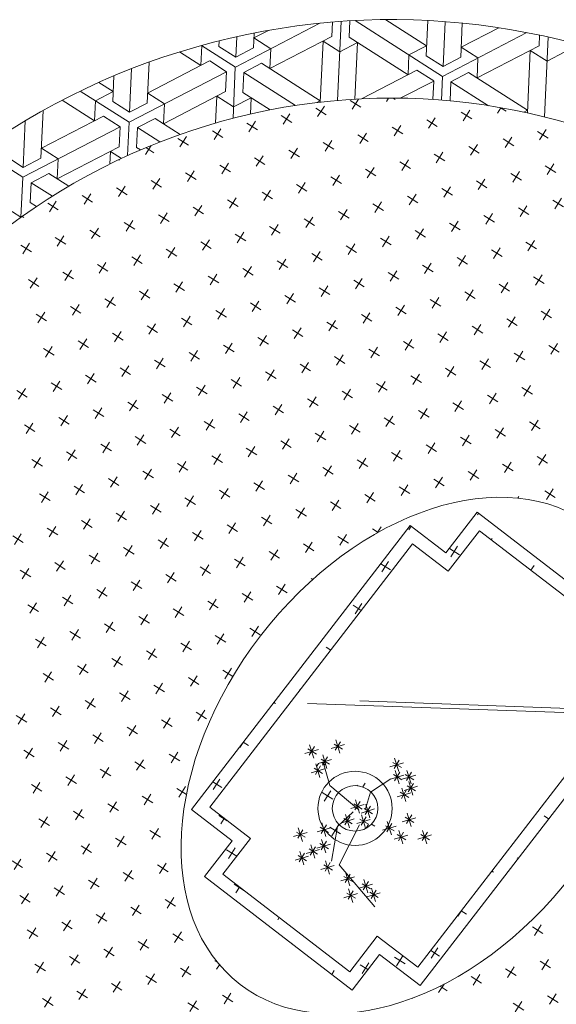
# Model space of a CAD drawing. Units: inches. Extents: x -4843 to -3402, y -164 to 3629.
# Tile 12 of 22: x -4506 to -4487, y 864 to 900. Entities that reach past the tile are written whole.
import ezdxf

# ---------------------------------------------------------------- set-up
doc = ezdxf.new("R2010")
doc.units = ezdxf.units.IN
doc.layers.add('furniture', color=6, linetype='Continuous', lineweight=18)

# ---------------------------------------------------------------- blocks, each defined once
blk = doc.blocks.new('A$C30AE1D3B')
for p, q in [((1385.7, 1569.4, -685.7), (1368.4, 1561.4, -685.7)), ((1381.1, 1556.7, -685.7), (1373, 1574, -685.7)), ((1436.3, 1551, -685.7), (1419.1, 1542.9, -685.7)), ((1431.7, 1538.3, -685.7), (1423.7, 1555.6, -685.7)), ((1362.7, 1506.1, -685.7), (1354.6, 1523.4, -685.7)), ((1367.3, 1518.8, -685.7), (1350, 1510.7, -685.7)), ((1413.3, 1487.7, -685.7), (1405.2, 1504.9, -685.7)), ((1417.9, 1500.3, -685.7), (1400.6, 1492.3, -685.7)), ((1468.5, 1481.9, -685.7), (1451.3, 1473.9, -685.7)), ((1463.9, 1469.3, -685.7), (1455.9, 1486.5, -685.7)), ((1348.8, 1468.1, -685.7), (1331.6, 1460.1, -685.7)), ((1344.2, 1455.5, -685.7), (1336.2, 1472.7, -685.7)), ((1519.2, 1463.5, -685.7), (1505.1, 1456.9, -685.7)), ((1512, 1456.3, -685.7), (1506.5, 1468.1, -685.7)), ((1557.3, 1449.2, -685.7), (1557.1, 1449.7, -685.7)), ((1013.2, 1248.8, -685.7), (1537, 1439.4, -685.7)), ((1537, 1439.4, -685.7), (1563.8, 1365.8, -685.7)), ((1494.9, 1402.8, -685.7), (1488.1, 1417.5, -685.7)), ((1038.9, 1236.8, -685.7), (1525.1, 1413.8, -685.7)), ((1500.7, 1412.9, -685.7), (1483.5, 1404.8, -685.7)), ((1525.1, 1413.8, -685.7), (1551.9, 1340.2, -685.7)), ((1423, 1376.7, -685.7), (1419, 1385.3, -685.7)), ((1551.4, 1394.4, -685.7), (1534.9, 1386.8, -685.7)), ((1546.8, 1381.8, -685.7), (1538.7, 1399, -685.7)), ((1563.8, 1365.8, -685.7), (1628.5, 1389.4, -685.7)), ((1628.5, 1389.4, -685.7), (1725.8, 1122.2, -685.7)), ((1431.7, 1380.6, -685.7), (1423.4, 1376.8, -685.7)), ((1602, 1376, -685.7), (1584.7, 1367.9, -685.7)), ((1597.4, 1363.3, -685.7), (1591.5, 1375.9, -685.7)), ((1307.4, 1354.2, -685.7), (1306.7, 1355.6, -685.7)), ((1551.9, 1340.2, -685.7), (1616.6, 1363.7, -685.7)), ((1616.6, 1363.7, -685.7), (1700.1, 1134.1, -685.7)), ((1351.1, 1350.5, -685.7), (1349.9, 1353.1, -685.7)), ((1641.9, 1352.6, -685.7), (1635.4, 1349.5, -685.7)), ((1238.3, 1322, -685.7), (1234.8, 1329.4, -685.7)), ((1525.7, 1294.5, -685.7), (1520, 1273.8, -685.7)), ((1542.7, 1217.2, -685.7), (1530.9, 1300.7, -685.7)), ((1804.5, 1302.3, -685.7), (1787.3, 1294.2, -685.7)), ((1799.9, 1289.6, -685.7), (1791.9, 1306.9, -685.7)), ((1533.2, 1281.3, -685.7), (1512.5, 1287.1, -685.7)), ((1529.1, 1286.7, -685.7), (1515.5, 1280.1, -685.7)), ((1525.6, 1277.8, -685.7), (1518.9, 1291.5, -685.7)), ((1668.1, 1280.7, -685.7), (1667.6, 1280.5, -685.7)), ((1855.2, 1283.9, -685.7), (1837.9, 1275.8, -685.7)), ((1850.5, 1271.2, -685.7), (1842.5, 1288.5, -685.7)), ((1536.2, 1263.8, -685.7), (1515.5, 1269.5, -685.7)), ((1532.1, 1269.2, -685.7), (1518.5, 1262.5, -685.7)), ((1528.6, 1260.3, -685.7), (1521.9, 1274, -685.7)), ((1528.7, 1277, -685.7), (1523, 1256.3, -685.7)), ((1563.4, 1263.5, -685.7), (1542.7, 1269.2, -685.7)), ((1559.3, 1268.9, -685.7), (1545.7, 1262.3, -685.7)), ((1555.8, 1260, -685.7), (1549.1, 1273.7, -685.7)), ((1555.9, 1276.7, -685.7), (1550.2, 1256, -685.7)), ((1419.9, 1248.5, -685.7), (1399.2, 1254.3, -685.7)), ((1415.8, 1254, -685.7), (1402.1, 1247.3, -685.7)), ((1412.3, 1245.1, -685.7), (1405.6, 1258.7, -685.7)), ((1412.4, 1261.8, -685.7), (1406.7, 1241.1, -685.7)), ((1545.9, 1236.1, -685.7), (1539.2, 1249.8, -685.7)), ((1546, 1252.8, -685.7), (1540.3, 1232.1, -685.7)), ((1786.1, 1251.6, -685.7), (1778.7, 1248.2, -685.7)), ((1381.8, 1022.6, -685.7), (1059.1, 1244.3, -685.7)), ((1450.6, 1229.2, -685.7), (1429.9, 1235, -685.7)), ((1446.5, 1234.7, -685.7), (1432.9, 1228, -685.7)), ((1443, 1225.7, -685.7), (1436.3, 1239.4, -685.7)), ((1443.1, 1242.4, -685.7), (1437.4, 1221.7, -685.7)), ((1553.5, 1239.5, -685.7), (1532.8, 1245.3, -685.7)), ((1549.4, 1245, -685.7), (1535.8, 1238.3, -685.7)), ((1666.4, 1237.9, -685.7), (1663, 1236.3, -685.7)), ((1781.5, 1239, -685.7), (1779.2, 1243.9, -685.7)), ((1832.1, 1220.6, -685.7), (1824.1, 1237.8, -685.7)), ((1425.9, 1213.4, -685.7), (1405.2, 1219.2, -685.7)), ((1421.8, 1218.9, -685.7), (1408.1, 1212.2, -685.7)), ((1418.3, 1210, -685.7), (1411.6, 1223.6, -685.7)), ((1418.4, 1226.7, -685.7), (1412.7, 1206, -685.7)), ((1450.8, 1221.5, -685.7), (1445, 1200.8, -685.7)), ((1562.5, 1221.5, -685.7), (1556.7, 1200.8, -685.7)), ((1836.7, 1233.2, -685.7), (1819.5, 1225.2, -685.7)), ((1882.7, 1202.1, -685.7), (1874.7, 1219.4, -685.7)), ((1451, 983.2, -685.7), (1128.3, 1204.9, -685.7)), ((1458.2, 1208.3, -685.7), (1437.5, 1214, -685.7)), ((1454.2, 1213.7, -685.7), (1440.5, 1207, -685.7)), ((1450.6, 1204.8, -685.7), (1444, 1218.5, -685.7)), ((1483.6, 1182.4, -685.7), (1542.7, 1217.2, -685.7)), ((1513.3, 1166.6, -685.7), (1549.3, 1206.3, -685.7)), ((1570, 1208.3, -685.7), (1549.3, 1214, -685.7)), ((1565.9, 1213.7, -685.7), (1552.2, 1207, -685.7)), ((1562.4, 1204.8, -685.7), (1555.7, 1218.5, -685.7)), ((1887.4, 1214.8, -685.7), (1870.1, 1206.7, -685.7)), ((1404.6, 1190.3, -685.7), (1398.8, 1169.6, -685.7)), ((1467.5, 1191.1, -685.7), (1465, 1196.5, -685.7)), ((1477.6, 1191.9, -685.7), (1471.6, 1189.1, -685.7)), ((1478.4, 1175.1, -685.7), (1471.7, 1188.8, -685.7)), ((1478.5, 1191.8, -685.7), (1472.8, 1171.1, -685.7)), ((1550, 1190.7, -685.7), (1544.3, 1170, -685.7)), ((1568.4, 1188.9, -685.7), (1562.7, 1168.2, -685.7)), ((1938, 1196.4, -685.7), (1920.7, 1188.3, -685.7)), ((1933.4, 1183.7, -685.7), (1925.3, 1201, -685.7)), ((1397.8, 1174.4, -685.7), (1377.1, 1180.2, -685.7)), ((1393.7, 1179.8, -685.7), (1380, 1173.2, -685.7)), ((1390.2, 1170.9, -685.7), (1383.5, 1184.6, -685.7)), ((1390.3, 1187.6, -685.7), (1384.6, 1166.9, -685.7)), ((1412, 1177.1, -685.7), (1391.3, 1182.8, -685.7)), ((1408, 1182.5, -685.7), (1394.3, 1175.8, -685.7)), ((1404.4, 1173.6, -685.7), (1397.8, 1187.3, -685.7)), ((1471.9, 1168.3, -685.7), (1451.2, 1174.1, -685.7)), ((1467.8, 1173.8, -685.7), (1454.2, 1167.1, -685.7)), ((1464.3, 1164.9, -685.7), (1457.6, 1178.6, -685.7)), ((1464.4, 1181.6, -685.7), (1458.7, 1160.9, -685.7)), ((1486, 1178.5, -685.7), (1465.3, 1184.3, -685.7)), ((1481.9, 1184, -685.7), (1468.2, 1177.3, -685.7)), ((1498.6, 1161.3, -685.7), (1492, 1174.9, -685.7)), ((1498.8, 1178, -685.7), (1493, 1157.3, -685.7)), ((1523.7, 1160.8, -685.7), (1515.6, 1178.1, -685.7)), ((1557.5, 1177.5, -685.7), (1536.8, 1183.2, -685.7)), ((1553.4, 1182.9, -685.7), (1539.7, 1176.2, -685.7)), ((1549.9, 1174, -685.7), (1543.2, 1187.7, -685.7)), ((1575.9, 1175.7, -685.7), (1555.2, 1181.5, -685.7)), ((1571.8, 1181.1, -685.7), (1558.2, 1174.5, -685.7)), ((1568.3, 1172.2, -685.7), (1561.6, 1185.9, -685.7)), ((1595.5, 1175.2, -685.7), (1574.8, 1181, -685.7)), ((1591.5, 1180.7, -685.7), (1577.8, 1174, -685.7)), ((1587.9, 1171.8, -685.7), (1581.3, 1185.4, -685.7)), ((1588.1, 1188.4, -685.7), (1582.3, 1167.7, -685.7)), ((1818.3, 1182.6, -685.7), (1801, 1174.5, -685.7)), ((1813.7, 1169.9, -685.7), (1805.6, 1187.2, -685.7)), ((1988.6, 1177.9, -685.7), (1971.4, 1169.9, -685.7)), ((1984, 1165.3, -685.7), (1976, 1182.5, -685.7)), ((1390.9, 1158.3, -685.7), (1370.2, 1164.1, -685.7)), ((1386.8, 1163.8, -685.7), (1373.2, 1157.1, -685.7)), ((1383.3, 1154.9, -685.7), (1376.6, 1168.6, -685.7)), ((1383.4, 1171.6, -685.7), (1377.7, 1150.9, -685.7)), ((1398.7, 1145.2, -685.7), (1392, 1158.9, -685.7)), ((1398.8, 1161.9, -685.7), (1393.1, 1141.2, -685.7)), ((1462.7, 1166.8, -685.7), (1442.7, 1148.9, -685.7)), ((1481.4, 1154, -685.7), (1460.7, 1159.8, -685.7)), ((1477.3, 1159.4, -685.7), (1463.6, 1152.8, -685.7)), ((1473.8, 1150.5, -685.7), (1467.1, 1164.2, -685.7)), ((1473.9, 1167.2, -685.7), (1468.2, 1146.5, -685.7)), ((1472.3, 1162.4, -685.7), (1489.6, 1107.5, -685.7)), ((1481.1, 1160.2, -685.7), (1513.3, 1166.6, -685.7)), ((1506.2, 1164.7, -685.7), (1485.5, 1170.5, -685.7)), ((1502.2, 1170.2, -685.7), (1488.5, 1163.5, -685.7)), ((1528.3, 1173.5, -685.7), (1511, 1165.4, -685.7)), ((1544, 1156.4, -685.7), (1523.3, 1162.2, -685.7)), ((1539.9, 1161.9, -685.7), (1526.2, 1155.2, -685.7)), ((1536.4, 1153, -685.7), (1529.7, 1166.7, -685.7)), ((1536.5, 1169.7, -685.7), (1530.7, 1149, -685.7)), ((1694, 1156.2, -685.7), (1685.9, 1173.4, -685.7)), ((1698.6, 1168.8, -685.7), (1689.1, 1164.4, -685.7)), ((1868.9, 1164.2, -685.7), (1851.7, 1156.1, -685.7)), ((1864.3, 1151.5, -685.7), (1856.3, 1168.8, -685.7)), ((2039.3, 1159.5, -685.7), (2022, 1151.5, -685.7)), ((2034.6, 1146.8, -685.7), (2026.6, 1164.1, -685.7)), ((1075.8, 875.5, -685.7), (975.3, 1151.6, -685.7)), ((1389.4, 1145.8, -685.7), (1383.7, 1125.1, -685.7)), ((1406.3, 1148.7, -685.7), (1385.6, 1154.5, -685.7)), ((1402.2, 1154.1, -685.7), (1388.5, 1147.5, -685.7)), ((1394.8, 1153.2, -685.7), (1393, 1152.4, -685.7)), ((1442.7, 1148.9, -685.7), (1405.6, 1148.7, -685.7)), ((1578.3, 1143.5, -685.7), (1557.6, 1149.3, -685.7)), ((1574.2, 1149, -685.7), (1560.6, 1142.3, -685.7)), ((1570.7, 1140.1, -685.7), (1564, 1153.7, -685.7)), ((1570.8, 1156.8, -685.7), (1565.1, 1136.1, -685.7)), ((1919.6, 1145.7, -685.7), (1902.3, 1137.7, -685.7)), ((1915, 1133.1, -685.7), (1906.9, 1150.3, -685.7)), ((1087.8, 901.2, -685.7), (1001, 1139.7, -685.7)), ((1396.9, 1132.6, -685.7), (1376.2, 1138.3, -685.7)), ((1392.8, 1138, -685.7), (1379.2, 1131.4, -685.7)), ((1389.3, 1129.1, -685.7), (1382.6, 1142.8, -685.7)), ((1448.2, 1136.1, -685.7), (1442, 1133.2, -685.7)), ((1454.6, 1128.6, -685.7), (1453.7, 1130.5, -685.7)), ((1700.1, 1134.1, -685.7), (1635.4, 1110.6, -685.7)), ((1799.9, 1132, -685.7), (1782.6, 1123.9, -685.7)), ((1795.3, 1119.3, -685.7), (1787.2, 1136.6, -685.7)), ((1965.6, 1114.6, -685.7), (1957.5, 1131.9, -685.7)), ((1509.8, 1122.8, -685.7), (1492.6, 1114.8, -685.7)), ((1505.2, 1110.2, -685.7), (1497.2, 1127.4, -685.7)), ((1725.8, 1122.2, -685.7), (1661.1, 1098.6, -685.7)), ((1680.2, 1118.2, -685.7), (1662.9, 1110.1, -685.7)), ((1675.6, 1105.5, -685.7), (1667.7, 1122.3, -685.7)), ((1850.5, 1113.5, -685.7), (1833.2, 1105.5, -685.7)), ((1845.9, 1100.9, -685.7), (1837.8, 1118.1, -685.7)), ((1970.2, 1127.3, -685.7), (1952.9, 1119.3, -685.7)), ((2016.2, 1096.2, -685.7), (2008.2, 1113.5, -685.7)), ((1489.6, 1107.5, -685.7), (1478.8, 1071.7, -685.7)), ((1635.4, 1110.6, -685.7), (1662.2, 1037, -685.7)), ((1661.1, 1098.6, -685.7), (1687.9, 1025, -685.7)), ((1896.5, 1082.4, -685.7), (1888.5, 1099.7, -685.7)), ((2020.8, 1108.9, -685.7), (2003.6, 1100.8, -685.7)), ((1495.6, 1072.1, -685.7), (1488.9, 1085.7, -685.7)), ((1495.7, 1088.8, -685.7), (1489.9, 1068.1, -685.7)), ((1776.8, 1068.7, -685.7), (1768.8, 1085.9, -685.7)), ((1901.1, 1095.1, -685.7), (1883.9, 1087, -685.7)), ((1450.2, 1057.2, -685.7), (1443.5, 1070.9, -685.7)), ((1450.3, 1073.9, -685.7), (1444.6, 1053.2, -685.7)), ((1486.7, 1069.5, -685.7), (1466, 1075.3, -685.7)), ((1482.6, 1075, -685.7), (1469, 1068.3, -685.7)), ((1479.1, 1066.1, -685.7), (1472.4, 1079.7, -685.7)), ((1479.2, 1082.8, -685.7), (1473.5, 1062.1, -685.7)), ((1481.5, 1071, -685.7), (1478.8, 1076.8, -685.7)), ((1503.2, 1075.5, -685.7), (1482.5, 1081.3, -685.7)), ((1499.1, 1081, -685.7), (1485.4, 1074.3, -685.7)), ((1491.1, 1072, -685.7), (1486.1, 1069.7, -685.7)), ((1657.1, 1054.9, -685.7), (1650.7, 1068.8, -685.7)), ((1781.4, 1081.3, -685.7), (1764.2, 1073.3, -685.7)), ((1951.8, 1076.7, -685.7), (1934.5, 1068.6, -685.7)), ((1947.2, 1064, -685.7), (1939.1, 1081.3, -685.7)), ((1457.8, 1060.7, -685.7), (1437.1, 1066.5, -685.7)), ((1453.7, 1066.1, -685.7), (1440, 1059.5, -685.7)), ((1487.8, 1042.1, -685.7), (1481.2, 1055.8, -685.7)), ((1488, 1058.8, -685.7), (1482.2, 1038.1, -685.7)), ((1661.7, 1067.6, -685.7), (1652.7, 1063.3, -685.7)), ((1832.1, 1062.9, -685.7), (1814.8, 1054.8, -685.7)), ((1827.5, 1050.2, -685.7), (1819.4, 1067.5, -685.7)), ((2002.4, 1058.2, -685.7), (1985.1, 1050.2, -685.7)), ((1997.8, 1045.6, -685.7), (1989.7, 1062.9, -685.7)), ((1495.4, 1045.6, -685.7), (1474.7, 1051.4, -685.7)), ((1491.4, 1051, -685.7), (1477.7, 1044.4, -685.7)), ((1882.7, 1044.5, -685.7), (1865.4, 1036.4, -685.7)), ((1878.1, 1031.8, -685.7), (1870, 1049.1, -685.7)), ((1687.9, 1025, -685.7), (1173, 837.6, -685.7)), ((1662.2, 1037, -685.7), (1184.9, 863.3, -685.7)), ((1763, 1030.7, -685.7), (1745.7, 1022.6, -685.7)), ((1758.4, 1018, -685.7), (1750.4, 1035.3, -685.7)), ((1933.3, 1026, -685.7), (1916.1, 1018, -685.7)), ((1928.7, 1013.4, -685.7), (1920.7, 1030.6, -685.7)), ((1643.3, 1016.9, -685.7), (1626.1, 1008.9, -685.7)), ((1637.6, 1006.7, -685.7), (1630.7, 1021.5, -685.7)), ((1813.6, 1012.3, -685.7), (1796.4, 1004.2, -685.7)), ((1809, 999.6, -685.7), (1801, 1016.9, -685.7)), ((1979.4, 995, -685.7), (1971.3, 1012.2, -685.7)), ((1053.9, 994.3, -685.7), (1046, 990.6, -685.7)), ((1693.9, 998.5, -685.7), (1676.7, 990.4, -685.7)), ((1689.3, 985.8, -685.7), (1682, 1001.6, -685.7)), ((1864.3, 993.8, -685.7), (1847, 985.8, -685.7)), ((1859.7, 981.2, -685.7), (1851.6, 998.4, -685.7)), ((1984, 1007.6, -685.7), (1966.7, 999.6, -685.7)), ((1565.7, 980.6, -685.7), (1561.6, 989.3, -685.7)), ((1574.3, 984.7, -685.7), (1564.2, 980, -685.7)), ((1744.6, 980.1, -685.7), (1727.3, 972, -685.7)), ((1740, 967.4, -685.7), (1731.9, 984.7, -685.7)), ((1910.3, 962.7, -685.7), (1902.2, 980, -685.7)), ((1790.6, 949, -685.7), (1782.6, 966.2, -685.7)), ((1914.9, 975.4, -685.7), (1897.6, 967.4, -685.7)), ((1450, 958.3, -685.7), (1449.4, 959.5, -685.7)), ((1493.8, 954.4, -685.7), (1492.5, 957.1, -685.7)), ((1670.9, 935.2, -685.7), (1662.9, 952.5, -685.7)), ((1795.2, 961.6, -685.7), (1777.9, 953.6, -685.7)), ((1965.5, 957, -685.7), (1948.3, 948.9, -685.7)), ((1960.9, 944.3, -685.7), (1952.9, 961.6, -685.7)), ((1380.9, 926.1, -685.7), (1377.5, 933.4, -685.7)), ((1675.5, 947.9, -685.7), (1658.3, 939.8, -685.7)), ((1721.5, 916.8, -685.7), (1713.5, 934, -685.7)), ((1845.8, 943.2, -685.7), (1828.6, 935.2, -685.7)), ((1841.2, 930.5, -685.7), (1833.2, 947.8, -685.7)), ((971.2, 903.2, -685.7), (963.1, 920.4, -685.7)), ((1080, 922.4, -685.7), (1078.2, 921.6, -685.7)), ((1161.4, 928, -685.7), (1087.8, 901.2, -685.7)), ((1184.9, 863.3, -685.7), (1161.4, 928, -685.7)), ((1601.9, 903, -685.7), (1593.8, 920.3, -685.7)), ((1726.2, 929.4, -685.7), (1708.9, 921.4, -685.7)), ((1896.5, 924.8, -685.7), (1879.2, 916.7, -685.7)), ((1891.9, 912.1, -685.7), (1883.8, 929.4, -685.7)), ((975.8, 915.8, -685.7), (958.5, 907.8, -685.7)), ((1146.1, 911.2, -685.7), (1128.9, 903.1, -685.7)), ((1141.1, 899.3, -685.7), (1133.5, 915.8, -685.7)), ((1316.4, 906.5, -685.7), (1299.2, 898.5, -685.7)), ((1311.8, 893.9, -685.7), (1305.6, 907.2, -685.7)), ((1606.5, 915.7, -685.7), (1589.2, 907.6, -685.7)), ((1776.8, 911, -685.7), (1759.5, 902.9, -685.7)), ((1772.2, 898.3, -685.7), (1764.1, 915.6, -685.7)), ((1011.7, 890.5, -685.7), (1009.2, 889.4, -685.7)), ((1149.4, 902.3, -685.7), (1075.8, 875.5, -685.7)), ((1173, 837.6, -685.7), (1149.4, 902.3, -685.7)), ((1657.1, 897.2, -685.7), (1639.8, 889.2, -685.7)), ((1652.5, 884.6, -685.7), (1644.4, 901.8, -685.7)), ((1827.4, 892.6, -685.7), (1810.2, 884.5, -685.7)), ((1822.8, 879.9, -685.7), (1814.8, 897.2, -685.7)), ((1077.1, 879, -685.7), (1074.9, 878, -685.7)), ((1247.4, 874.3, -685.7), (1230.1, 866.3, -685.7)), ((1242.2, 862.8, -685.7), (1234.7, 878.9, -685.7)), ((1537.4, 883.5, -685.7), (1520.1, 875.4, -685.7)), ((1532.8, 870.8, -685.7), (1525.2, 887.1, -685.7)), ((1707.7, 878.8, -685.7), (1690.5, 870.7, -685.7)), ((1703.1, 866.1, -685.7), (1695.1, 883.4, -685.7)), ((1878, 874.1, -685.7), (1860.8, 866.1, -685.7)), ((1873.4, 861.5, -685.7), (1865.4, 878.8, -685.7)), ((957.4, 865.2, -685.7), (940.1, 857.2, -685.7)), ((952.8, 852.5, -685.7), (944.7, 869.8, -685.7)), ((1588, 865, -685.7), (1570.8, 857, -685.7)), ((1583.4, 852.4, -685.7), (1575.4, 869.6, -685.7)), ((1758.4, 860.4, -685.7), (1741.1, 852.3, -685.7)), ((1753.7, 847.7, -685.7), (1745.7, 865, -685.7)), ((1008, 846.8, -685.7), (990.7, 838.7, -685.7)), ((1003.4, 834.1, -685.7), (995.3, 851.4, -685.7)), ((1468.3, 851.2, -685.7), (1451.1, 843.2, -685.7)), ((1463.7, 838.6, -685.7), (1455.7, 855.9, -685.7)), ((1638.7, 846.6, -685.7), (1621.4, 838.5, -685.7)), ((1634.1, 833.9, -685.7), (1626, 851.2, -685.7)), ((1804.4, 829.3, -685.7), (1796.3, 846.5, -685.7)), ((1058.6, 828.4, -685.7), (1041.4, 820.3, -685.7)), ((1054, 815.7, -685.7), (1046, 833, -685.7)), ((1178.3, 842.1, -685.7), (1172.3, 839.3, -685.7)), ((1519, 832.8, -685.7), (1501.7, 824.8, -685.7)), ((1514.4, 820.2, -685.7), (1506.3, 837.4, -685.7)), ((1689.3, 828.2, -685.7), (1672, 820.1, -685.7)), ((1684.7, 815.5, -685.7), (1676.6, 832.8, -685.7)), ((1809, 841.9, -685.7), (1791.7, 833.9, -685.7)), ((1855, 810.9, -685.7), (1847, 828.1, -685.7)), ((938.9, 814.6, -685.7), (921.7, 806.5, -685.7)), ((934.3, 801.9, -685.7), (926.3, 819.2, -685.7)), ((1104.7, 797.3, -685.7), (1096.6, 814.5, -685.7)), ((1221.4, 820.2, -685.7), (1211.7, 815.6, -685.7)), ((1224.3, 811, -685.7), (1220, 820.3, -685.7)), ((1344, 824.8, -685.7), (1342.8, 827.4, -685.7)), ((1399.3, 819, -685.7), (1382, 811, -685.7)), ((1394.7, 806.4, -685.7), (1386.6, 823.7, -685.7)), ((1569.6, 814.4, -685.7), (1552.3, 806.3, -685.7)), ((1565, 801.7, -685.7), (1556.9, 819, -685.7)), ((1735.3, 797.1, -685.7), (1727.3, 814.3, -685.7)), ((1859.6, 823.5, -685.7), (1842.4, 815.5, -685.7)), ((985, 783.5, -685.7), (976.9, 800.8, -685.7)), ((1109.3, 809.9, -685.7), (1092, 801.9, -685.7)), ((1279.6, 805.3, -685.7), (1262.3, 797.2, -685.7)), ((1275, 792.6, -685.7), (1266.9, 809.9, -685.7)), ((1449.9, 800.6, -685.7), (1432.6, 792.6, -685.7)), ((1445.3, 788, -685.7), (1437.3, 805.2, -685.7)), ((1615.6, 783.3, -685.7), (1607.6, 800.6, -685.7)), ((1739.9, 809.7, -685.7), (1722.7, 801.7, -685.7)), ((989.6, 796.1, -685.7), (972.3, 788.1, -685.7)), ((1159.9, 791.5, -685.7), (1142.6, 783.4, -685.7)), ((1155.3, 778.8, -685.7), (1147.2, 796.1, -685.7)), ((1330.2, 786.8, -685.7), (1313, 778.8, -685.7)), ((1325.6, 774.2, -685.7), (1317.6, 791.4, -685.7)), ((1495.9, 769.5, -685.7), (1487.9, 786.8, -685.7)), ((1620.2, 796, -685.7), (1603, 787.9, -685.7)), ((1790.6, 791.3, -685.7), (1773.3, 783.3, -685.7)), ((1786, 778.6, -685.7), (1777.9, 795.9, -685.7)), ((915.9, 751.3, -685.7), (907.8, 768.6, -685.7)), ((1040.2, 777.7, -685.7), (1022.9, 769.7, -685.7)), ((1035.6, 765.1, -685.7), (1027.5, 782.3, -685.7)), ((1210.5, 773.1, -685.7), (1193.3, 765, -685.7)), ((1205.9, 760.4, -685.7), (1197.9, 777.7, -685.7)), ((1380.8, 768.4, -685.7), (1363.6, 760.4, -685.7)), ((1376.2, 755.8, -685.7), (1368.2, 773, -685.7)), ((1500.5, 782.2, -685.7), (1483.3, 774.1, -685.7)), ((1546.6, 751.1, -685.7), (1538.5, 768.4, -685.7)), ((1670.9, 777.5, -685.7), (1653.6, 769.5, -685.7)), ((1666.3, 764.9, -685.7), (1658.2, 782.1, -685.7)), ((1841.2, 772.9, -685.7), (1823.9, 764.8, -685.7)), ((1836.6, 760.2, -685.7), (1828.5, 777.5, -685.7)), ((920.5, 763.9, -685.7), (903.2, 755.9, -685.7)), ((1090.8, 759.3, -685.7), (1073.6, 751.2, -685.7)), ((1086.2, 746.6, -685.7), (1078.2, 763.9, -685.7)), ((1261.2, 754.6, -685.7), (1243.9, 746.6, -685.7)), ((1256.5, 742, -685.7), (1248.5, 759.2, -685.7)), ((1426.9, 737.3, -685.7), (1418.8, 754.6, -685.7)), ((1551.2, 763.8, -685.7), (1533.9, 755.7, -685.7)), ((1721.5, 759.1, -685.7), (1704.2, 751.1, -685.7)), ((1716.9, 746.4, -685.7), (1708.8, 763.7, -685.7)), ((971.1, 745.5, -685.7), (953.9, 737.5, -685.7)), ((966.5, 732.9, -685.7), (958.5, 750.1, -685.7)), ((1141.5, 740.9, -685.7), (1124.2, 732.8, -685.7)), ((1136.9, 728.2, -685.7), (1128.8, 745.5, -685.7)), ((1307.2, 723.5, -685.7), (1299.1, 740.8, -685.7)), ((1431.5, 750, -685.7), (1414.2, 741.9, -685.7)), ((1601.8, 745.3, -685.7), (1584.5, 737.3, -685.7)), ((1597.2, 732.7, -685.7), (1589.1, 749.9, -685.7)), ((1772.1, 740.7, -685.7), (1754.9, 732.6, -685.7)), ((1767.5, 728, -685.7), (1759.5, 745.3, -685.7)), ((851.4, 731.7, -685.7), (834.2, 723.7, -685.7)), ((846.8, 719.1, -685.7), (838.8, 736.3, -685.7)), ((1021.8, 727.1, -685.7), (1004.5, 719, -685.7)), ((1017.2, 714.4, -685.7), (1009.1, 731.7, -685.7)), ((1192.1, 722.4, -685.7), (1174.8, 714.4, -685.7)), ((1187.5, 709.8, -685.7), (1179.4, 727, -685.7)), ((1311.8, 736.2, -685.7), (1294.5, 728.2, -685.7)), ((1357.8, 705.1, -685.7), (1349.8, 722.4, -685.7)), ((1482.1, 731.6, -685.7), (1464.8, 723.5, -685.7)), ((1477.5, 718.9, -685.7), (1469.5, 736.2, -685.7)), ((1652.4, 726.9, -685.7), (1635.2, 718.8, -685.7)), ((1647.8, 714.2, -685.7), (1639.8, 731.5, -685.7)), ((902.1, 713.3, -685.7), (884.8, 705.3, -685.7)), ((897.5, 700.7, -685.7), (889.4, 717.9, -685.7)), ((1072.4, 708.7, -685.7), (1055.1, 700.6, -685.7)), ((1067.8, 696, -685.7), (1059.7, 713.3, -685.7)), ((1238.1, 691.3, -685.7), (1230.1, 708.6, -685.7)), ((1362.4, 717.8, -685.7), (1345.2, 709.7, -685.7)), ((1532.7, 713.1, -685.7), (1515.5, 705.1, -685.7)), ((1528.1, 700.5, -685.7), (1520.1, 717.7, -685.7)), ((1703.1, 708.5, -685.7), (1685.8, 700.4, -685.7)), ((1698.5, 695.8, -685.7), (1690.4, 713.1, -685.7)), ((952.7, 694.9, -685.7), (935.4, 686.8, -685.7)), ((948.1, 682.2, -685.7), (940.1, 699.5, -685.7)), ((1118.4, 677.6, -685.7), (1110.4, 694.8, -685.7)), ((1242.7, 704, -685.7), (1225.5, 696, -685.7)), ((1413.1, 699.4, -685.7), (1395.8, 691.3, -685.7)), ((1408.4, 686.7, -685.7), (1400.4, 704, -685.7)), ((1583.4, 694.7, -685.7), (1566.1, 686.6, -685.7)), ((1578.8, 682, -685.7), (1570.7, 699.3, -685.7)), ((1749.1, 677.4, -685.7), (1741, 694.7, -685.7)), ((833, 681.1, -685.7), (815.8, 673.1, -685.7)), ((828.4, 668.5, -685.7), (820.4, 685.7, -685.7)), ((998.7, 663.8, -685.7), (990.7, 681.1, -685.7)), ((1123, 690.2, -685.7), (1105.8, 682.2, -685.7)), ((1293.4, 685.6, -685.7), (1276.1, 677.5, -685.7)), ((1288.8, 672.9, -685.7), (1280.7, 690.2, -685.7)), ((1463.7, 680.9, -685.7), (1446.4, 672.9, -685.7)), ((1459.1, 668.3, -685.7), (1451, 685.5, -685.7)), ((1629.4, 663.6, -685.7), (1621.4, 680.9, -685.7)), ((1753.7, 690, -685.7), (1736.4, 682, -685.7)), ((883.6, 662.7, -685.7), (866.4, 654.6, -685.7)), ((879, 650, -685.7), (871, 667.3, -685.7)), ((1003.3, 676.5, -685.7), (986.1, 668.4, -685.7)), ((1049.4, 645.4, -685.7), (1041.3, 662.6, -685.7)), ((1173.7, 671.8, -685.7), (1156.4, 663.7, -685.7)), ((1169.1, 659.1, -685.7), (1161, 676.4, -685.7)), ((1344, 667.1, -685.7), (1326.7, 659.1, -685.7)), ((1339.4, 654.5, -685.7), (1331.3, 671.8, -685.7)), ((1514.3, 662.5, -685.7), (1497.1, 654.4, -685.7)), ((1509.7, 649.8, -685.7), (1501.7, 667.1, -685.7)), ((1634, 676.3, -685.7), (1616.7, 668.2, -685.7)), ((1680, 645.2, -685.7), (1672, 662.4, -685.7)), ((929.7, 631.6, -685.7), (921.6, 648.9, -685.7)), ((1054, 658, -685.7), (1036.7, 650, -685.7)), ((1224.3, 653.4, -685.7), (1207, 645.3, -685.7)), ((1219.7, 640.7, -685.7), (1211.6, 658, -685.7)), ((1394.6, 648.7, -685.7), (1377.4, 640.7, -685.7)), ((1390, 636.1, -685.7), (1382, 653.3, -685.7)), ((1560.3, 631.4, -685.7), (1552.3, 648.7, -685.7)), ((1684.6, 657.8, -685.7), (1667.4, 649.8, -685.7)), ((810, 617.8, -685.7), (801.9, 635.1, -685.7)), ((934.3, 644.3, -685.7), (917, 636.2, -685.7)), ((1104.6, 639.6, -685.7), (1087.3, 631.5, -685.7)), ((1100, 626.9, -685.7), (1091.9, 644.2, -685.7)), ((1274.9, 634.9, -685.7), (1257.7, 626.9, -685.7)), ((1270.3, 622.3, -685.7), (1262.3, 639.6, -685.7)), ((1440.6, 617.6, -685.7), (1432.6, 634.9, -685.7)), ((1564.9, 644.1, -685.7), (1547.7, 636, -685.7)), ((1735.3, 639.4, -685.7), (1718, 631.4, -685.7)), ((1730.7, 626.8, -685.7), (1722.6, 644, -685.7)), ((814.6, 630.5, -685.7), (797.3, 622.4, -685.7)), ((984.9, 625.8, -685.7), (967.6, 617.8, -685.7)), ((980.3, 613.2, -685.7), (972.3, 630.4, -685.7)), ((1155.2, 621.2, -685.7), (1138, 613.1, -685.7)), ((1150.6, 608.5, -685.7), (1142.6, 625.8, -685.7)), ((1321, 603.9, -685.7), (1312.9, 621.1, -685.7)), ((1445.3, 630.3, -685.7), (1428, 622.2, -685.7)), ((1615.6, 625.6, -685.7), (1598.3, 617.6, -685.7)), ((1611, 613, -685.7), (1602.9, 630.2, -685.7)), ((865.2, 612, -685.7), (848, 604, -685.7)), ((860.6, 599.4, -685.7), (852.6, 616.7, -685.7)), ((1035.5, 607.4, -685.7), (1018.3, 599.3, -685.7)), ((1030.9, 594.7, -685.7), (1022.9, 612, -685.7)), ((1205.9, 602.7, -685.7), (1188.6, 594.7, -685.7)), ((1201.3, 590.1, -685.7), (1193.2, 607.3, -685.7)), ((1325.6, 616.5, -685.7), (1308.3, 608.5, -685.7)), ((1371.6, 585.4, -685.7), (1363.5, 602.7, -685.7)), ((1495.9, 611.9, -685.7), (1478.6, 603.8, -685.7)), ((1491.3, 599.2, -685.7), (1483.2, 616.5, -685.7)), ((1666.2, 607.2, -685.7), (1648.9, 599.2, -685.7)), ((1661.6, 594.5, -685.7), (1653.6, 611.8, -685.7)), ((915.9, 593.6, -685.7), (898.6, 585.6, -685.7)), ((911.2, 581, -685.7), (903.2, 598.2, -685.7)), ((1086.2, 589, -685.7), (1068.9, 580.9, -685.7)), ((1081.6, 576.3, -685.7), (1073.5, 593.6, -685.7)), ((1251.9, 571.7, -685.7), (1243.8, 588.9, -685.7)), ((1376.2, 598.1, -685.7), (1358.9, 590, -685.7)), ((1546.5, 593.4, -685.7), (1529.3, 585.4, -685.7)), ((1541.9, 580.8, -685.7), (1533.9, 598, -685.7)), ((1716.8, 588.8, -685.7), (1699.6, 580.7, -685.7)), ((1712.2, 576.1, -685.7), (1704.2, 593.4, -685.7)), ((796.2, 579.8, -685.7), (778.9, 571.8, -685.7)), ((791.6, 567.2, -685.7), (783.5, 584.5, -685.7)), ((966.5, 575.2, -685.7), (949.2, 567.1, -685.7)), ((961.9, 562.5, -685.7), (953.8, 579.8, -685.7)), ((1132.2, 557.9, -685.7), (1124.2, 575.1, -685.7)), ((1256.5, 584.3, -685.7), (1239.2, 576.3, -685.7)), ((1426.8, 579.7, -685.7), (1409.6, 571.6, -685.7)), ((1422.2, 567, -685.7), (1414.2, 584.3, -685.7)), ((1597.2, 575, -685.7), (1579.9, 567, -685.7)), ((1592.5, 562.3, -685.7), (1584.5, 579.6, -685.7)), ((846.8, 561.4, -685.7), (829.5, 553.4, -685.7)), ((842.2, 548.8, -685.7), (834.1, 566, -685.7)), ((1017.1, 556.8, -685.7), (999.9, 548.7, -685.7)), ((1012.5, 544.1, -685.7), (1004.5, 561.4, -685.7)), ((1136.8, 570.5, -685.7), (1119.5, 562.5, -685.7)), ((1307.1, 565.9, -685.7), (1289.9, 557.8, -685.7)), ((1302.5, 553.2, -685.7), (1294.5, 570.5, -685.7)), ((1477.5, 561.2, -685.7), (1460.2, 553.2, -685.7)), ((1472.9, 548.6, -685.7), (1464.8, 565.8, -685.7)), ((1643.2, 543.9, -685.7), (1635.1, 561.2, -685.7)), ((727.1, 547.6, -685.7), (709.8, 539.6, -685.7)), ((722.5, 535, -685.7), (714.4, 552.2, -685.7)), ((897.4, 543, -685.7), (880.2, 534.9, -685.7)), ((892.8, 530.3, -685.7), (884.8, 547.6, -685.7)), ((1063.1, 525.7, -685.7), (1055.1, 542.9, -685.7)), ((1187.4, 552.1, -685.7), (1170.2, 544.1, -685.7)), ((1182.8, 539.5, -685.7), (1174.8, 556.7, -685.7)), ((1357.8, 547.5, -685.7), (1340.5, 539.4, -685.7)), ((1353.2, 534.8, -685.7), (1345.1, 552.1, -685.7)), ((1528.1, 542.8, -685.7), (1510.8, 534.7, -685.7)), ((1523.5, 530.1, -685.7), (1515.4, 547.4, -685.7)), ((1647.8, 556.6, -685.7), (1630.5, 548.5, -685.7)), ((1693.8, 525.5, -685.7), (1685.8, 542.8, -685.7)), ((777.7, 529.2, -685.7), (760.5, 521.2, -685.7)), ((773.1, 516.6, -685.7), (765.1, 533.8, -685.7)), ((943.4, 511.9, -685.7), (935.4, 529.2, -685.7)), ((1067.7, 538.3, -685.7), (1050.5, 530.3, -685.7)), ((1238.1, 533.7, -685.7), (1220.8, 525.6, -685.7)), ((1233.5, 521, -685.7), (1225.4, 538.3, -685.7)), ((1408.4, 529, -685.7), (1391.1, 521, -685.7)), ((1403.8, 516.4, -685.7), (1395.7, 533.6, -685.7)), ((1574.1, 511.7, -685.7), (1566.1, 529, -685.7)), ((1698.4, 538.1, -685.7), (1681.2, 530.1, -685.7)), ((823.8, 498.1, -685.7), (815.7, 515.4, -685.7)), ((948.1, 524.6, -685.7), (930.8, 516.5, -685.7)), ((1118.4, 519.9, -685.7), (1101.1, 511.9, -685.7)), ((1113.8, 507.2, -685.7), (1105.7, 524.5, -685.7)), ((1288.7, 515.3, -685.7), (1271.4, 507.2, -685.7)), ((1284.1, 502.6, -685.7), (1276, 519.9, -685.7)), ((1454.4, 497.9, -685.7), (1446.4, 515.2, -685.7)), ((1578.7, 524.4, -685.7), (1561.5, 516.3, -685.7)), ((708.7, 497, -685.7), (691.4, 489, -685.7)), ((704.1, 484.4, -685.7), (696, 501.6, -685.7)), ((828.4, 510.8, -685.7), (811.1, 502.7, -685.7)), ((874.4, 479.7, -685.7), (866.3, 497, -685.7)), ((998.7, 506.1, -685.7), (981.4, 498.1, -685.7)), ((994.1, 493.5, -685.7), (986, 510.7, -685.7)), ((1169, 501.5, -685.7), (1151.7, 493.4, -685.7)), ((1164.4, 488.8, -685.7), (1156.4, 506.1, -685.7)), ((1339.3, 496.8, -685.7), (1322.1, 488.8, -685.7)), ((1334.7, 484.2, -685.7), (1326.7, 501.4, -685.7)), ((1459, 510.6, -685.7), (1441.8, 502.5, -685.7)), ((1505.1, 479.5, -685.7), (1497, 496.8, -685.7)), ((1629.4, 505.9, -685.7), (1612.1, 497.9, -685.7)), ((1624.7, 493.3, -685.7), (1616.7, 510.6, -685.7)), ((754.7, 465.9, -685.7), (746.6, 483.2, -685.7)), ((879, 492.4, -685.7), (861.7, 484.3, -685.7)), ((1049.3, 487.7, -685.7), (1032.1, 479.7, -685.7)), ((1044.7, 475, -685.7), (1036.7, 492.3, -685.7)), ((1219.6, 483, -685.7), (1202.4, 475, -685.7)), ((1215, 470.4, -685.7), (1207, 487.7, -685.7)), ((1385.4, 465.7, -685.7), (1377.3, 483, -685.7)), ((1509.7, 492.2, -685.7), (1492.4, 484.1, -685.7)), ((759.3, 478.6, -685.7), (742, 470.5, -685.7)), ((929.6, 473.9, -685.7), (912.4, 465.9, -685.7)), ((925, 461.3, -685.7), (917, 478.5, -685.7)), ((1100, 469.3, -685.7), (1082.7, 461.2, -685.7)), ((1095.3, 456.6, -685.7), (1087.3, 473.9, -685.7)), ((1265.7, 452, -685.7), (1257.6, 469.2, -685.7)), ((1390, 478.4, -685.7), (1372.7, 470.3, -685.7)), ((1560.3, 473.7, -685.7), (1543, 465.7, -685.7)), ((1555.7, 461.1, -685.7), (1547.6, 478.3, -685.7)), ((809.9, 460.2, -685.7), (792.7, 452.1, -685.7)), ((805.3, 447.5, -685.7), (797.3, 464.8, -685.7)), ((980.3, 455.5, -685.7), (963, 447.4, -685.7)), ((975.7, 442.8, -685.7), (967.6, 460.1, -685.7)), ((1146, 438.2, -685.7), (1137.9, 455.5, -685.7)), ((1270.3, 464.6, -685.7), (1253, 456.6, -685.7)), ((1440.6, 460, -685.7), (1423.3, 451.9, -685.7)), ((1436, 447.3, -685.7), (1427.9, 464.6, -685.7)), ((1610.9, 455.3, -685.7), (1593.7, 447.3, -685.7)), ((1606.3, 442.7, -685.7), (1598.3, 459.9, -685.7)), ((690.2, 446.4, -685.7), (673, 438.3, -685.7)), ((685.6, 433.7, -685.7), (677.6, 451, -685.7)), ((860.6, 441.7, -685.7), (843.3, 433.7, -685.7)), ((856, 429.1, -685.7), (847.9, 446.3, -685.7)), ((1030.9, 437.1, -685.7), (1013.6, 429, -685.7)), ((1026.3, 424.4, -685.7), (1018.2, 441.7, -685.7)), ((1150.6, 450.8, -685.7), (1133.3, 442.8, -685.7)), ((1196.6, 419.8, -685.7), (1188.6, 437, -685.7)), ((1320.9, 446.2, -685.7), (1303.6, 438.1, -685.7)), ((1316.3, 433.5, -685.7), (1308.3, 450.8, -685.7)), ((1491.2, 441.5, -685.7), (1474, 433.5, -685.7)), ((1486.6, 428.9, -685.7), (1478.6, 446.1, -685.7)), ((740.9, 427.9, -685.7), (723.6, 419.9, -685.7)), ((736.3, 415.3, -685.7), (728.2, 432.6, -685.7)), ((911.2, 423.3, -685.7), (893.9, 415.2, -685.7)), ((906.6, 410.6, -685.7), (898.5, 427.9, -685.7)), ((1076.9, 406, -685.7), (1068.9, 423.2, -685.7)), ((1201.2, 432.4, -685.7), (1184, 424.4, -685.7)), ((1371.5, 427.8, -685.7), (1354.3, 419.7, -685.7)), ((1366.9, 415.1, -685.7), (1358.9, 432.4, -685.7)), ((1541.9, 423.1, -685.7), (1524.6, 415.1, -685.7)), ((1537.3, 410.5, -685.7), (1529.2, 427.7, -685.7)), ((594.9, 320.7, -685.7), (665, 420.8, -685.7)), ((791.5, 409.5, -685.7), (774.2, 401.5, -685.7)), ((786.9, 396.9, -685.7), (778.8, 414.1, -685.7)), ((957.2, 392.2, -685.7), (949.2, 409.5, -685.7)), ((1081.5, 418.6, -685.7), (1064.3, 410.6, -685.7)), ((1251.8, 414, -685.7), (1234.6, 405.9, -685.7)), ((1247.2, 401.3, -685.7), (1239.2, 418.6, -685.7)), ((1422.2, 409.3, -685.7), (1404.9, 401.3, -685.7)), ((1417.6, 396.7, -685.7), (1409.5, 413.9, -685.7)), ((1587.9, 392, -685.7), (1579.8, 409.3, -685.7)), ((683.8, 401.6, -685.7), (628.9, 323.1, -685.7)), ((726.4, 301.4, -685.7), (681.3, 398.1, -685.7)), ((687.9, 397.5, -685.7), (681.3, 398, -685.7)), ((837.5, 378.4, -685.7), (829.5, 395.7, -685.7)), ((961.8, 404.9, -685.7), (944.6, 396.8, -685.7)), ((1132.2, 400.2, -685.7), (1114.9, 392.2, -685.7)), ((1127.5, 387.6, -685.7), (1119.5, 404.8, -685.7)), ((1302.5, 395.6, -685.7), (1285.2, 387.5, -685.7)), ((1297.9, 382.9, -685.7), (1289.8, 400.2, -685.7)), ((1468.2, 378.2, -685.7), (1460.1, 395.5, -685.7)), ((1592.5, 404.7, -685.7), (1575.2, 396.6, -685.7)), ((714.1, 372.8, -685.7), (709.8, 381.9, -685.7)), ((722.4, 377.3, -685.7), (713.6, 373.2, -685.7)), ((842.1, 391.1, -685.7), (824.9, 383, -685.7)), ((888.2, 360, -685.7), (880.1, 377.3, -685.7)), ((1012.5, 386.4, -685.7), (995.2, 378.4, -685.7)), ((1007.9, 373.8, -685.7), (999.8, 391, -685.7)), ((1182.8, 381.8, -685.7), (1165.5, 373.7, -685.7)), ((1178.2, 369.1, -685.7), (1170.1, 386.4, -685.7)), ((1353.1, 377.1, -685.7), (1335.8, 369.1, -685.7)), ((1348.5, 364.5, -685.7), (1340.5, 381.7, -685.7)), ((1472.8, 390.9, -685.7), (1455.5, 382.9, -685.7)), ((1518.8, 359.8, -685.7), (1510.8, 377.1, -685.7)), ((768.5, 346.2, -685.7), (760.4, 363.5, -685.7)), ((892.8, 372.7, -685.7), (875.5, 364.6, -685.7)), ((1063.1, 368, -685.7), (1045.8, 360, -685.7)), ((1058.5, 355.4, -685.7), (1050.4, 372.6, -685.7)), ((1233.4, 363.4, -685.7), (1216.2, 355.3, -685.7)), ((1228.8, 350.7, -685.7), (1220.8, 368, -685.7)), ((1399.1, 346, -685.7), (1391.1, 363.3, -685.7)), ((1523.4, 372.5, -685.7), (1506.2, 364.4, -685.7)), ((616, 350.8, -685.7), (585.6, 353.4, -685.7)), ((615.9, 350.8, -685.7), (628.8, 323.2, -685.7)), ((728, 360.3, -685.7), (756.7, 298.7, -685.7)), ((773.1, 358.9, -685.7), (755.8, 350.8, -685.7)), ((943.4, 354.2, -685.7), (926.1, 346.2, -685.7)), ((938.8, 341.6, -685.7), (930.7, 358.8, -685.7)), ((1113.7, 349.6, -685.7), (1096.5, 341.5, -685.7)), ((1109.1, 336.9, -685.7), (1101.1, 354.2, -685.7)), ((1279.4, 332.3, -685.7), (1271.4, 349.5, -685.7)), ((1403.7, 358.7, -685.7), (1386.5, 350.7, -685.7)), ((1574.1, 354, -685.7), (1556.8, 346, -685.7)), ((1569.5, 341.4, -685.7), (1561.4, 358.7, -685.7)), ((823.7, 340.5, -685.7), (806.4, 332.4, -685.7)), ((819.1, 327.8, -685.7), (811.1, 345.1, -685.7)), ((994, 335.8, -685.7), (976.8, 327.8, -685.7)), ((989.4, 323.1, -685.7), (981.4, 340.4, -685.7)), ((1164.4, 331.2, -685.7), (1147.1, 323.1, -685.7)), ((1159.8, 318.5, -685.7), (1151.7, 335.8, -685.7)), ((1284.1, 344.9, -685.7), (1266.8, 336.9, -685.7)), ((1330.1, 313.8, -685.7), (1322, 331.1, -685.7)), ((1454.4, 340.3, -685.7), (1437.1, 332.2, -685.7)), ((1449.8, 327.6, -685.7), (1441.7, 344.9, -685.7)), ((604.4, 311.3, -685.7), (613.7, 324.5, -685.7)), ((613.7, 324.5, -685.7), (719.9, 315.2, -685.7)), ((756.7, 298.7, -685.7), (773.6, 322.8, -685.7)), ((874.3, 322, -685.7), (857.1, 314, -685.7)), ((869.7, 309.4, -685.7), (861.7, 326.6, -685.7)), ((1044.7, 317.4, -685.7), (1027.4, 309.3, -685.7)), ((1040.1, 304.7, -685.7), (1032, 322, -685.7)), ((1210.4, 300.1, -685.7), (1202.3, 317.3, -685.7)), ((1334.7, 326.5, -685.7), (1317.4, 318.4, -685.7)), ((1505, 321.8, -685.7), (1487.7, 313.8, -685.7)), ((1500.4, 309.2, -685.7), (1492.4, 326.5, -685.7)), ((702.5, 290.2, -685.7), (719.9, 315.2, -685.7)), ((756.7, 298.7, -685.7), (726.4, 301.3, -685.7)), ((763.2, 284.9, -685.7), (784.1, 314.7, -685.7)), ((778.4, 283.6, -685.7), (794.7, 306.9, -685.7)), ((925, 303.6, -685.7), (907.7, 295.6, -685.7)), ((920.4, 290.9, -685.7), (912.3, 308.2, -685.7)), ((1090.7, 286.3, -685.7), (1082.6, 303.6, -685.7)), ((1215, 312.7, -685.7), (1197.7, 304.7, -685.7)), ((1385.3, 308.1, -685.7), (1368.1, 300, -685.7)), ((1380.7, 295.4, -685.7), (1372.7, 312.7, -685.7)), ((763.2, 284.9, -685.7), (618.7, 297.5, -685.7)), ((702.4, 290.2, -685.7), (715.3, 262.6, -685.7)), ((971, 272.5, -685.7), (962.9, 289.8, -685.7)), ((1095.3, 298.9, -685.7), (1078, 290.9, -685.7)), ((1265.6, 294.3, -685.7), (1248.4, 286.2, -685.7)), ((1261, 281.6, -685.7), (1253, 298.9, -685.7)), ((1435.9, 289.6, -685.7), (1418.7, 281.6, -685.7)), ((1431.3, 277, -685.7), (1423.3, 294.2, -685.7)), ((724.1, 275.1, -685.7), (694.2, 232.4, -685.7)), ((715.2, 216.4, -685.7), (754.4, 272.4, -685.7)), ((754.4, 272.4, -685.7), (724.1, 275.1, -685.7)), ((754.4, 272.4, -685.7), (767.3, 244.8, -685.7)), ((763.2, 284.9, -685.7), (830.1, 141.4, -685.7)), ((778.3, 283.6, -685.7), (791.2, 255.9, -685.7)), ((835.6, 278.5, -685.7), (778.4, 283.6, -685.7)), ((844.9, 272.5, -685.7), (843.3, 276, -685.7)), ((855.9, 271.4, -685.7), (850.6, 268.9, -685.7)), ((975.6, 285.2, -685.7), (958.3, 277.1, -685.7)), ((1021.6, 254.1, -685.7), (1013.6, 271.4, -685.7)), ((1145.9, 280.5, -685.7), (1128.7, 272.5, -685.7)), ((1141.3, 267.9, -685.7), (1133.3, 285.1, -685.7)), ((1316.3, 275.9, -685.7), (1299, 267.8, -685.7)), ((1311.6, 263.2, -685.7), (1303.6, 280.5, -685.7)), ((1486.6, 271.2, -685.7), (1469.3, 263.2, -685.7)), ((1482, 258.6, -685.7), (1473.9, 275.8, -685.7)), ((651, 268.2, -685.7), (715.3, 262.6, -685.7)), ((791.2, 255.9, -685.7), (886.1, 247.6, -685.7)), ((901.9, 240.3, -685.7), (893.9, 257.6, -685.7)), ((1026.2, 266.7, -685.7), (1009, 258.7, -685.7)), ((1196.6, 262.1, -685.7), (1179.3, 254, -685.7)), ((1192, 249.4, -685.7), (1183.9, 266.7, -685.7)), ((1366.9, 257.4, -685.7), (1349.6, 249.4, -685.7)), ((1362.3, 244.8, -685.7), (1354.2, 262, -685.7)), ((767.3, 244.8, -685.7), (736.6, 200.9, -685.7)), ((789, 229.6, -685.7), (806.4, 254.6, -685.7)), ((851.5, 157.9, -685.7), (806.4, 254.6, -685.7)), ((894.8, 242.7, -685.7), (845.1, 171.7, -685.7)), ((906.5, 253, -685.7), (890.1, 245.3, -685.7)), ((1076.9, 248.3, -685.7), (1059.6, 240.3, -685.7)), ((1072.3, 235.7, -685.7), (1064.2, 252.9, -685.7)), ((1247.2, 243.7, -685.7), (1229.9, 235.6, -685.7)), ((1242.6, 231, -685.7), (1234.5, 248.3, -685.7)), ((1412.9, 226.4, -685.7), (1404.9, 243.6, -685.7)), ((789.8, 165.4, -685.7), (758.6, 232.3, -685.7)), ((788.9, 229.6, -685.7), (758.6, 232.3, -685.7)), ((848.8, 131.1, -685.7), (918.2, 230.1, -685.7)), ((957.2, 234.5, -685.7), (939.9, 226.5, -685.7)), ((952.6, 221.9, -685.7), (944.5, 239.1, -685.7)), ((1127.5, 229.9, -685.7), (1110.2, 221.8, -685.7)), ((1122.9, 217.2, -685.7), (1114.8, 234.5, -685.7)), ((1293.2, 212.6, -685.7), (1285.2, 229.8, -685.7)), ((1417.5, 239, -685.7), (1400.3, 231, -685.7)), ((942, 218.1, -685.7), (888.3, 141.5, -685.7)), ((985.8, 119.7, -685.7), (940.8, 216.4, -685.7)), ((946.6, 215.8, -685.7), (940.8, 216.3, -685.7)), ((1007.8, 216.1, -685.7), (990.5, 208.1, -685.7)), ((1003.2, 203.5, -685.7), (995.2, 220.7, -685.7)), ((1178.1, 211.5, -685.7), (1160.9, 203.4, -685.7)), ((1173.5, 198.8, -685.7), (1165.5, 216.1, -685.7)), ((1297.8, 225.2, -685.7), (1280.6, 217.2, -685.7)), ((1343.9, 194.1, -685.7), (1335.8, 211.4, -685.7)), ((1468.2, 220.6, -685.7), (1450.9, 212.5, -685.7)), ((1463.5, 207.9, -685.7), (1455.5, 225.2, -685.7)), ((976.6, 202, -685.7), (1016.2, 117, -685.7)), ((1058.4, 197.7, -685.7), (1041.2, 189.6, -685.7)), ((1053.8, 185, -685.7), (1045.8, 202.3, -685.7)), ((1224.2, 180.4, -685.7), (1216.1, 197.6, -685.7)), ((1348.5, 206.8, -685.7), (1331.2, 198.8, -685.7)), ((1033.7, 142, -685.7), (1012.7, 187, -685.7)), ((1104.5, 166.6, -685.7), (1096.4, 183.9, -685.7)), ((1228.8, 193, -685.7), (1211.5, 185, -685.7)), ((1399.1, 188.4, -685.7), (1381.8, 180.3, -685.7)), ((1394.5, 175.7, -685.7), (1386.4, 193, -685.7)), ((875.4, 169.1, -685.7), (845.1, 171.7, -685.7)), ((875.4, 169.1, -685.7), (888.3, 141.5, -685.7)), ((1022.7, 103.2, -685.7), (1067.6, 167.4, -685.7)), ((1041.6, 176.2, -685.7), (1027.3, 155.8, -685.7)), ((1109.1, 179.3, -685.7), (1091.8, 171.2, -685.7)), ((1279.4, 174.6, -685.7), (1262.1, 166.6, -685.7)), ((1274.8, 161.9, -685.7), (1266.7, 179.2, -685.7)), ((1449.7, 169.9, -685.7), (1432.5, 161.9, -685.7)), ((1445.1, 157.3, -685.7), (1437.1, 174.6, -685.7)), ((837.2, 137.4, -685.7), (851.5, 157.9, -685.7)), ((1057.6, 153.1, -685.7), (1027.2, 155.8, -685.7)), ((1057.6, 153.2, -685.7), (1070.5, 125.5, -685.7)), ((1094.1, 159.2, -685.7), (1070.5, 125.5, -685.7)), ((1159.7, 160.8, -685.7), (1142.4, 152.8, -685.7)), ((1155.1, 148.2, -685.7), (1147, 165.4, -685.7)), ((1330, 156.2, -685.7), (1312.8, 148.1, -685.7)), ((1325.4, 143.5, -685.7), (1317.4, 160.8, -685.7)), ((860.6, 124.8, -685.7), (873.1, 142.8, -685.7)), ((873.1, 142.8, -685.7), (979.4, 133.5, -685.7)), ((1016.2, 117, -685.7), (1033.7, 142, -685.7)), ((1168, 103.7, -685.7), (1148.9, 144.8, -685.7)), ((1181.2, 137.9, -685.7), (1198.4, 101.1, -685.7)), ((1210.3, 142.4, -685.7), (1195.2, 135.3, -685.7)), ((1203.8, 133.8, -685.7), (1197.7, 147, -685.7)), ((1380.7, 137.7, -685.7), (1363.4, 129.7, -685.7)), ((1376.1, 125.1, -685.7), (1368, 142.4, -685.7)), ((961.9, 108.5, -685.7), (979.4, 133.5, -685.7)), ((1037.8, 101.9, -685.7), (1055.3, 126.9, -685.7)), ((1055.3, 126.8, -685.7), (1161.6, 117.5, -685.7)), ((1198.4, 101.1, -685.7), (1215.9, 126.1, -685.7)), ((1204.8, 87.3, -685.7), (1234.2, 129.1, -685.7)), ((1215.9, 126.1, -685.7), (1213, 132.3, -685.7)), ((1244.2, 127.8, -685.7), (1252.7, 109.6, -685.7)), ((1249, 127.2, -685.7), (1248.3, 128.6, -685.7)), ((1263.8, 125.5, -685.7), (1252.7, 109.6, -685.7)), ((1350.2, 87.8, -685.7), (1334.9, 120.5, -685.7)), ((1387, 71.3, -685.7), (1422.2, 121.6, -685.7)), ((1419.8, 121.4, -685.7), (1418.6, 123.9, -685.7)), ((1422, 121.3, -685.7), (1419.8, 121.4, -685.7)), ((1422, 121.3, -685.7), (1434.9, 93.7, -685.7)), ((1022.6, 103.2, -685.7), (878, 115.9, -685.7)), ((961.9, 108.5, -685.7), (974.8, 80.9, -685.7)), ((1016.2, 117, -685.7), (985.8, 119.7, -685.7)), ((1144.1, 92.6, -685.7), (1161.6, 117.6, -685.7)), ((1220, 85.9, -685.7), (1237.5, 110.9, -685.7)), ((1237.5, 110.9, -685.7), (1343.8, 101.6, -685.7)), ((1364.3, 120, -685.7), (1380.6, 85.2, -685.7)), ((1380.6, 85.1, -685.7), (1398.1, 110.1, -685.7)), ((1398.1, 110.1, -685.7), (1393.3, 120.4, -685.7)), ((983.6, 93.4, -685.7), (970.5, 74.7, -685.7)), ((1013.9, 90.7, -685.7), (983.5, 93.4, -685.7)), ((996, 65.1, -685.7), (1013.9, 90.7, -685.7)), ((1013.9, 90.7, -685.7), (1026.8, 63.1, -685.7)), ((1022.6, 103.2, -685.7), (1048.6, 47.5, -685.7)), ((1204.8, 87.3, -685.7), (1037.8, 101.9, -685.7)), ((1037.8, 101.9, -685.7), (1050.7, 74.3, -685.7)), ((1144.1, 92.6, -685.7), (1157, 65, -685.7)), ((1198.4, 101.1, -685.7), (1168, 103.7, -685.7)), ((1326.3, 76.6, -685.7), (1343.8, 101.6, -685.7)), ((949.6, 83.1, -685.7), (974.8, 80.9, -685.7)), ((1165.7, 77.4, -685.7), (1129.8, 26.1, -685.7)), ((1196.1, 74.8, -685.7), (1165.7, 77.4, -685.7)), ((1204.8, 87.3, -685.7), (1242.2, 7.2, -685.7)), ((1220, 86, -685.7), (1232.9, 58.3, -685.7)), ((1387, 71.3, -685.7), (1220, 85.9, -685.7)), ((1326.3, 76.7, -685.7), (1339.2, 49, -685.7)), ((1380.6, 85.1, -685.7), (1350.2, 87.8, -685.7)), ((1026.8, 63.1, -685.7), (1021.9, 56.1, -685.7)), ((1048.4, 48, -685.7), (1065.9, 72.9, -685.7)), ((1050.7, 74.2, -685.7), (1157, 64.9, -685.7)), ((1082.3, 37.8, -685.7), (1065.9, 72.9, -685.7)), ((1157.9, 20.2, -685.7), (1196.1, 74.8, -685.7)), ((1196.1, 74.8, -685.7), (1209, 47.2, -685.7)), ((1347.9, 61.5, -685.7), (1306, 1.7, -685.7)), ((1378.3, 58.8, -685.7), (1347.9, 61.5, -685.7)), ((1387, 71.3, -685.7), (1419.7, 1.3, -685.7)), ((1048.4, 47.9, -685.7), (1046.7, 48.1, -685.7)), ((1209, 47.2, -685.7), (1186.5, 15, -685.7)), ((1230.6, 32, -685.7), (1248.1, 57, -685.7)), ((1232.9, 58.3, -685.7), (1339.2, 49, -685.7)), ((1272.8, 4.1, -685.7), (1248.1, 57, -685.7)), ((1337.4, 0.4, -685.7), (1378.3, 58.9, -685.7)), ((1378.3, 58.9, -685.7), (1391.1, 31.2, -685.7)), ((1211.2, 11.2, -685.7), (1200.2, 34.7, -685.7)), ((1230.6, 32, -685.7), (1200.2, 34.7, -685.7))]:
    blk.add_line(p, q)
for radius in [56.7, 34.8]:
    blk.add_circle((1475.8, 1157.4, -685.7), radius)
for radius, start, end in [(1089.4, 168.469, 338.3492), (969.4, 168.0362, 346.8505)]:
    blk.add_arc((1366.9, 1089.4, -685.7), radius, start, end)
blk.add_ellipse((1353.7, 1139.3, -685.7), major_axis=(414.6, 150.9), ratio=0.680002)

msp = doc.modelspace()

# ---------------------------------------------------------------- block references
at = {"layer": 'furniture', "xscale": 0.0242257431082848, "yscale": 0.0242257431082848, "zscale": 0.0242257431082848, "rotation": 212.4298414976532}
msp.add_blockref('A$C30AE1D3B', (-4478.842, 914.005, -463.669), dxfattribs=at)

doc.saveas('drawing.dxf')
